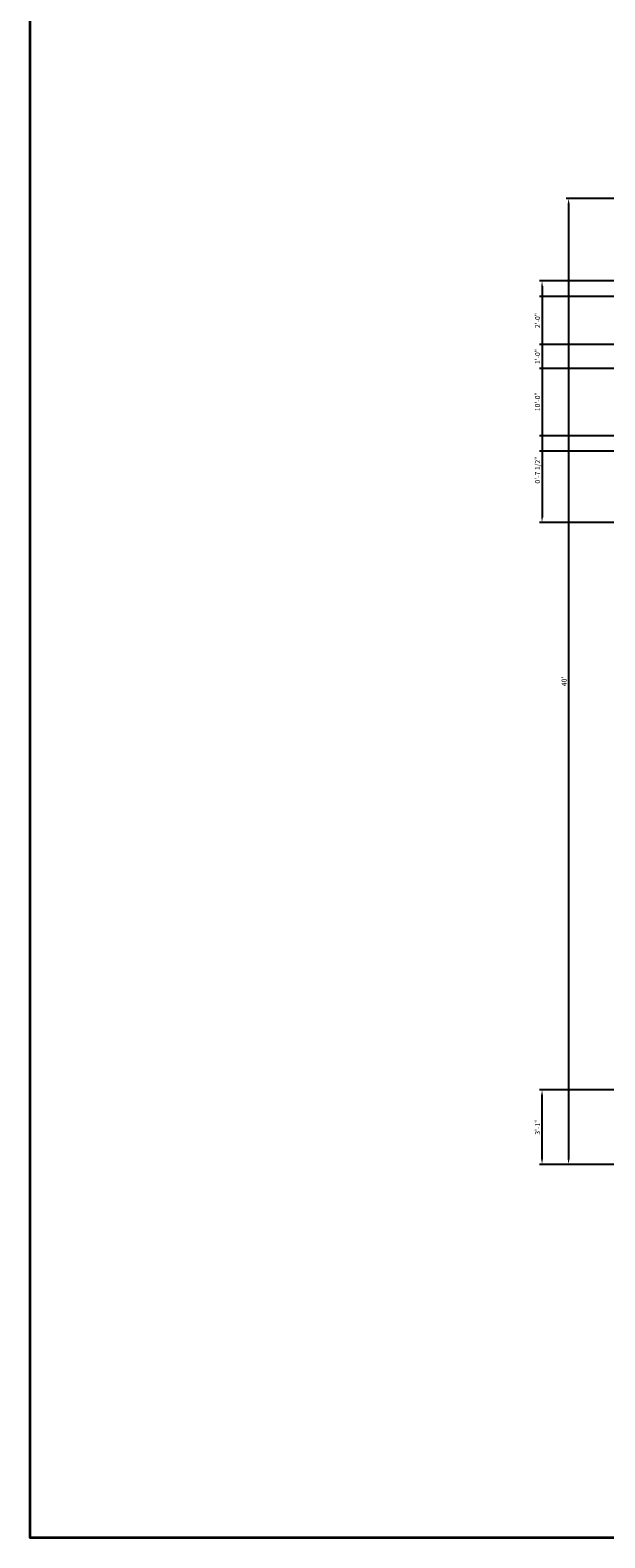
# Model space of a CAD drawing. Units: inches. Extents: x 2020 to 7901, y 1581 to 3943.
# Tile 1 of 17: x 2020 to 2305, y 1581 to 2330. Entities that reach past the tile are written whole.
import ezdxf

# ---------------------------------------------------------------- set-up
doc = ezdxf.new("R2010")
doc.units = ezdxf.units.IN
doc.layers.add('A-ANNO-DIMS', color=2, linetype='Continuous', lineweight=18)
doc.layers.add('A-ANNO-TTLB', color=7, linetype='Continuous', lineweight=35)
doc.styles.get("Standard").update_dxf_attribs({"font": 'arial.ttf'})
doc.dimstyles.new('ISO-25', dxfattribs={"dimtxt": 2.5, "dimasz": 2.5, "dimexe": 1.25, "dimexo": 0.625, "dimtad": 1, "dimdec": 1, "dimlunit": 3, "dimtxsty": 'Standard', "dimcen": 2.5, "dimadec": 0, "dimazin": 0, "dimtfac": 1, "dimtdec": 1, "dimtmove": 0, "dimatfit": 3, "dimfxl": 1, "dimarcsym": 0})

# ---------------------------------------------------------------- blocks, each defined once
blk = doc.blocks.new('*D4')
at = {"layer": 'A-ANNO-DIMS', "color": 0, "lineweight": -2, "transparency": 16777216}
for p, q in [((2358.34, 2246.34), (2285.83, 2246.34)), ((2287.08, 2243.84), (2287.08, 1768.84)), ((2358.34, 1766.34), (2285.83, 1766.34))]:
    blk.add_line(p, q, dxfattribs=at)
at = {"layer": 'A-ANNO-DIMS', "color": 0, "transparency": 16777216}
for points in [[(2286.66, 2243.84), (2287.49, 2243.84), (2287.08, 2246.34)], [(2286.66, 1768.84), (2287.49, 1768.84), (2287.08, 1766.34)]]:
    blk.add_solid(points, dxfattribs=at)
at = {"layer": 'DEFPOINTS', "color": 0, "transparency": 16777216}
for p in [(2358.96, 2246.34), (2287.08, 1766.34), (2358.96, 1766.34)]:
    blk.add_point(p, dxfattribs=at)
at = {"layer": 'A-ANNO-DIMS', "color": 0, "transparency": 16777216, "insert": (2285.18, 2006.34), "char_height": 2.5, "attachment_point": 5, "rotation": 90}
blk.add_mtext("40'", dxfattribs=at)
blk = doc.blocks.new('*D41')
at = {"layer": 'A-ANNO-DIMS', "color": 0, "lineweight": -2, "transparency": 16777216}
for p, q in [((2400.34, 2197.7), (2272.67, 2197.7)), ((2273.92, 2195.2), (2273.92, 2176.2)), ((2400.34, 2173.7), (2272.67, 2173.7))]:
    blk.add_line(p, q, dxfattribs=at)
at = {"layer": 'A-ANNO-DIMS', "color": 0, "transparency": 16777216}
for points in [[(2273.5, 2195.2), (2274.33, 2195.2), (2273.92, 2197.7)], [(2273.5, 2176.2), (2274.33, 2176.2), (2273.92, 2173.7)]]:
    blk.add_solid(points, dxfattribs=at)
at = {"layer": 'DEFPOINTS', "color": 0, "transparency": 16777216}
for p in [(2400.96, 2197.7), (2273.92, 2173.7), (2400.96, 2173.7)]:
    blk.add_point(p, dxfattribs=at)
at = {"layer": 'A-ANNO-DIMS', "color": 0, "transparency": 16777216, "insert": (2272.01, 2185.7), "char_height": 2.5, "attachment_point": 5, "rotation": 90}
blk.add_mtext('2\'-0"', dxfattribs=at)
blk = doc.blocks.new('*D42')
at = {"layer": 'A-ANNO-DIMS', "color": 0, "lineweight": -2, "transparency": 16777216}
for p, q in [((2536.48, 1803.34), (2272.67, 1803.34)), ((2273.92, 1768.84), (2273.92, 1800.84)), ((2536.48, 1766.34), (2272.67, 1766.34))]:
    blk.add_line(p, q, dxfattribs=at)
at = {"layer": 'A-ANNO-DIMS', "color": 0, "transparency": 16777216}
for points in [[(2273.5, 1800.84), (2274.33, 1800.84), (2273.92, 1803.34)], [(2273.5, 1768.84), (2274.33, 1768.84), (2273.92, 1766.34)]]:
    blk.add_solid(points, dxfattribs=at)
at = {"layer": 'DEFPOINTS', "color": 0, "transparency": 16777216}
for p in [(2273.92, 1803.34), (2537.1, 1803.34), (2537.1, 1766.34)]:
    blk.add_point(p, dxfattribs=at)
at = {"layer": 'A-ANNO-DIMS', "color": 0, "transparency": 16777216, "insert": (2272.01, 1784.84), "char_height": 2.5, "attachment_point": 5, "rotation": 90}
blk.add_mtext('3\'-1"', dxfattribs=at)
blk = doc.blocks.new('*D106')
at = {"layer": 'A-ANNO-DIMS', "color": 0, "lineweight": -2, "transparency": 16777216}
for p, q in [((2476.99, 2205.34), (2272.67, 2205.34)), ((2273.92, 2202.84), (2273.92, 2087.84)), ((2479.18, 2085.34), (2272.67, 2085.34))]:
    blk.add_line(p, q, dxfattribs=at)
at = {"layer": 'A-ANNO-DIMS', "color": 0, "transparency": 16777216}
for points in [[(2273.5, 2202.84), (2274.33, 2202.84), (2273.92, 2205.34)], [(2273.5, 2087.84), (2274.33, 2087.84), (2273.92, 2085.34)]]:
    blk.add_solid(points, dxfattribs=at)
at = {"layer": 'DEFPOINTS', "color": 0, "transparency": 16777216}
for p in [(2477.61, 2205.34), (2273.92, 2085.34), (2479.8, 2085.34)]:
    blk.add_point(p, dxfattribs=at)
at = {"layer": 'A-ANNO-DIMS', "color": 0, "transparency": 16777216, "insert": (2272.01, 2145.34), "char_height": 2.5, "attachment_point": 5, "rotation": 90}
blk.add_mtext('10\'-0"', dxfattribs=at)
blk = doc.blocks.new('*D111')
at = {"layer": 'A-ANNO-DIMS', "color": 0, "lineweight": -2, "transparency": 16777216}
for p, q in [((2540.34, 2128.34), (2272.67, 2128.34)), ((2540.34, 2120.73), (2272.67, 2120.73)), ((2273.92, 2125.84), (2273.92, 2123.23)), ((2273.92, 2120.73), (2273.92, 2104.51))]:
    blk.add_line(p, q, dxfattribs=at)
at = {"layer": 'A-ANNO-DIMS', "color": 0, "transparency": 16777216}
for points in [[(2273.5, 2125.84), (2274.33, 2125.84), (2273.92, 2128.34)], [(2273.5, 2123.23), (2274.33, 2123.23), (2273.92, 2120.73)]]:
    blk.add_solid(points, dxfattribs=at)
at = {"layer": 'DEFPOINTS', "color": 0, "transparency": 16777216}
for p in [(2540.96, 2128.34), (2273.92, 2120.73), (2540.96, 2120.73)]:
    blk.add_point(p, dxfattribs=at)
at = {"layer": 'A-ANNO-DIMS', "color": 0, "transparency": 16777216, "insert": (2272, 2111.37), "char_height": 2.5, "attachment_point": 5, "rotation": 90}
blk.add_mtext('0\'-7 1/2"', dxfattribs=at)
blk = doc.blocks.new('*D118')
at = {"layer": 'A-ANNO-DIMS', "color": 0, "lineweight": -2, "transparency": 16777216}
for p, q in [((2400.34, 2173.7), (2272.67, 2173.7)), ((2273.92, 2171.2), (2273.92, 2164.37)), ((2400.34, 2161.87), (2272.67, 2161.87))]:
    blk.add_line(p, q, dxfattribs=at)
at = {"layer": 'A-ANNO-DIMS', "color": 0, "transparency": 16777216}
for points in [[(2273.5, 2171.2), (2274.33, 2171.2), (2273.92, 2173.7)], [(2273.5, 2164.37), (2274.33, 2164.37), (2273.92, 2161.87)]]:
    blk.add_solid(points, dxfattribs=at)
at = {"layer": 'DEFPOINTS', "color": 0, "transparency": 16777216}
for p in [(2400.96, 2173.7), (2273.92, 2161.87), (2400.96, 2161.87)]:
    blk.add_point(p, dxfattribs=at)
at = {"layer": 'A-ANNO-DIMS', "color": 0, "transparency": 16777216, "insert": (2272.01, 2167.79), "char_height": 2.5, "attachment_point": 5, "rotation": 90}
blk.add_mtext('1\'-0"', dxfattribs=at)

msp = doc.modelspace()

# ---------------------------------------------------------------- linework, layer by layer
at = {"layer": 'A-ANNO-TTLB'}
msp.add_lwpolyline([(2019.8, 3067.25), (4199.03, 3067.25), (4199.03, 1580.73), (2019.8, 1580.73)], close=True, dxfattribs=at)

# ---------------------------------------------------------------- dimensions: what is measured, and where the dimension line sits
at = {"layer": 'A-ANNO-DIMS'}
for base, p1, p2, override, picture, middle in [((2287.08, 1766.34), (2358.96, 2246.34), (2358.96, 1766.34), {"dimclrd": 0, "dimclre": 0, "dimclrt": 0}, '*D4', (2285.18, 2006.34)), ((2273.92, 2085.34), (2477.61, 2205.34), (2479.8, 2085.34), {"dimdec": 1, "dimlfac": 1, "dimrnd": 0, "dimzin": 1, "dimdsep": 46, "dimlunit": 4, "dimfrac": 2}, '*D106', (2272.01, 2145.34)), ((2273.92, 2173.7), (2400.96, 2197.7), (2400.96, 2173.7), {"dimdec": 1, "dimlfac": 1, "dimrnd": 0, "dimzin": 1, "dimdsep": 46, "dimlunit": 4, "dimfrac": 2}, '*D41', (2272.01, 2185.7)), ((2273.92, 2161.87), (2400.96, 2173.7), (2400.96, 2161.87), {"dimdec": 1, "dimlfac": 1, "dimrnd": 0, "dimzin": 1, "dimdsep": 46, "dimlunit": 4, "dimfrac": 2}, '*D118', (2272.01, 2167.79)), ((2273.92, 2120.73), (2540.96, 2128.34), (2540.96, 2120.73), {"dimdec": 1, "dimlfac": 1, "dimrnd": 0, "dimzin": 1, "dimdsep": 46, "dimlunit": 4, "dimfrac": 2}, '*D111', (2272, 2111.37)), ((2273.92, 1803.34), (2537.1, 1766.34), (2537.1, 1803.34), {"dimdec": 1, "dimlfac": 1, "dimrnd": 0, "dimzin": 1, "dimdsep": 46, "dimlunit": 4, "dimfrac": 2}, '*D42', (2272.01, 1784.84))]:
    dim = msp.add_linear_dim(base=base, p1=p1, p2=p2, angle=90, dimstyle='ISO-25', override=override, dxfattribs=at)
    dim.commit()
    dim.dimension.update_dxf_attribs({"geometry": picture, "text_midpoint": middle})

doc.saveas('drawing.dxf')
